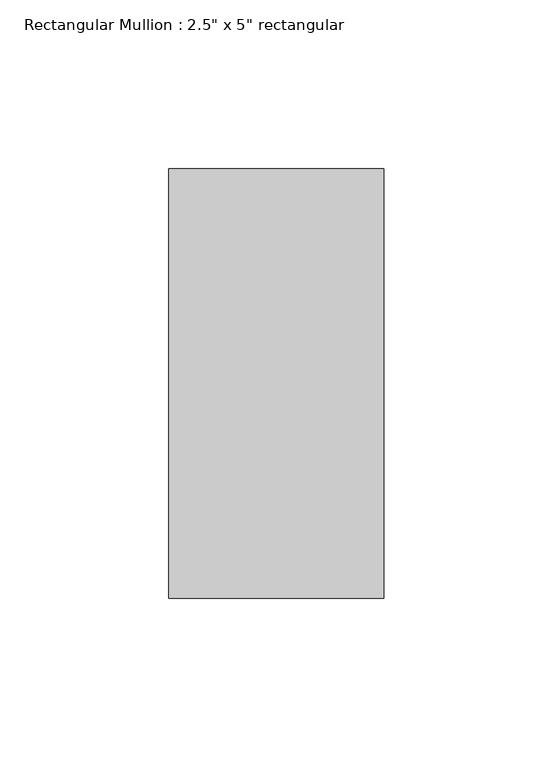
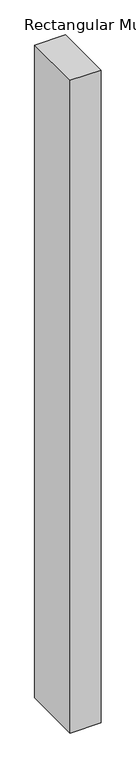
"""IFC4 building model written with IfcOpenShell, lengths in millimetres: member geometry."""

from ifc_helpers import new_model, si_unit, frame, origin, place, context, project, spatial, polyline, outline, extrude, source, transform, mapped, element, save


def member_5cae1c76(model_context):
    return source(origin(), model_context, "Body", "SweptSolid", [
        extrude(outline(polyline([(31.75, 63.5), (31.75, -63.5), (-31.75, -63.5), (-31.75, 63.5), (31.75, 63.5)])), frame((0.0, 0.0, -1425.0105727), z_axis=(0.0, 0.0, 1.0), x_axis=(1.0, 0.0, 0.0)), (0.0, 0.0, 1.0), 1425.0105727),
    ])


if __name__ == "__main__":
    model = new_model("IFC4")
    model_context = context("Model", 3, world=origin())
    ifc_project = project(units=[si_unit("LENGTHUNIT", "METRE", prefix="MILLI")], contexts=[model_context])
    site = spatial("IfcSite", under=ifc_project)
    building = spatial("IfcBuilding", under=site)
    placement = place(None, origin())
    member_shape = member_5cae1c76(model_context)
    element("IfcMember", 1, ObjectType="Rectangular Mullion : 2.5\" x 5\" rectangular", at=placement, inside=building, context=model_context, shape_type="MappedRepresentation", body=[
        mapped(member_shape, transform((0.0, 0.0, 0.0), x_axis=(1.0, 0.0, 0.0), y_axis=(0.0, 1.0, 0.0), z_axis=(0.0, 0.0, 1.0))),
    ])
    save(model, "model.ifc")

# Revit data of these elements
# Type "Rectangular Mullion : 2.5\" x 5\" rectangular"
#   built-in parameter 1007304 = 0.416667 (stored number, unit not read)
#   built-in parameter 1007301 = 0.104167 (stored number, unit not read)
#   built-in parameter 1007300 = 0.104167 (stored number, unit not read)
# Element 1 (IfcMember, "Rectangular Mullion : 2.5\" x 5\" rectangular")
#   Materials on its faces: "Aluminum"
# Materials
#   "Aluminum": class "Metal", colour RGB 247 247 247, transparency 0, Description = "Aluminum 6061", Cost = 0
